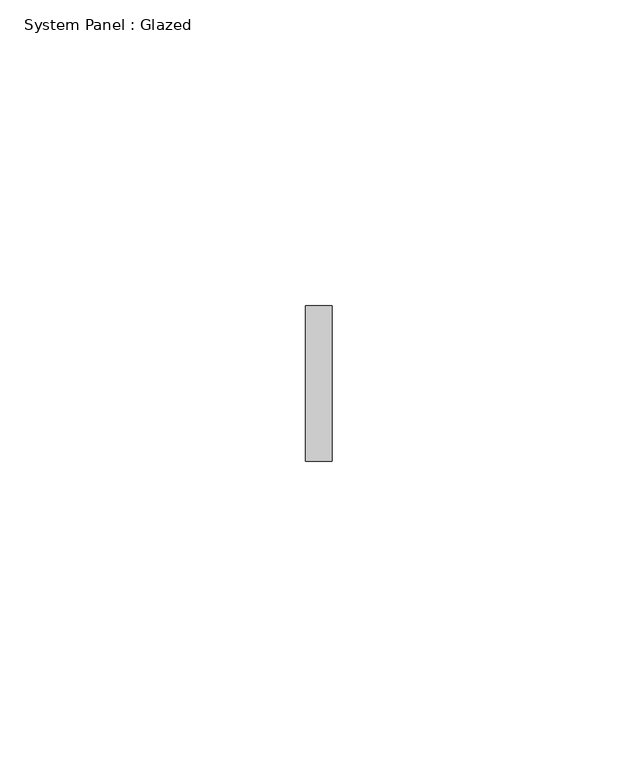
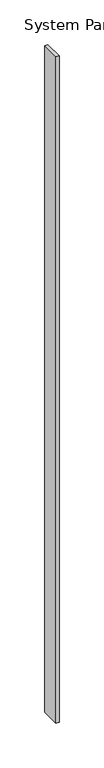
"""IFC4 building model written with IfcOpenShell, lengths in millimetres: plate geometry, System Panel : Glazed."""

from ifc_helpers import new_model, si_unit, origin, origin_with_axes, place, context, project, spatial, polyline, outline, extrude, source, transform, mapped, element, save


def system_panel_glazed_ffe51582(model_context):
    return source(origin(), model_context, "Body", "SweptSolid", [
        extrude(outline(polyline([(2.1789755, 19.05), (-2.1789755, 19.05), (-2.1789755, 44.45), (2.1789755, 44.45), (2.1789755, 19.05)])), origin_with_axes(), (0.0, 0.0, 1.0), 914.4),
    ])


if __name__ == "__main__":
    model = new_model("IFC4")
    model_context = context("Model", 3, world=origin())
    ifc_project = project(units=[si_unit("LENGTHUNIT", "METRE", prefix="MILLI")], contexts=[model_context])
    site = spatial("IfcSite", under=ifc_project)
    building = spatial("IfcBuilding", under=site)
    placement = place(None, origin())
    system_panel_glazed_shape = system_panel_glazed_ffe51582(model_context)
    element("IfcPlate", 1, ObjectType="System Panel : Glazed", at=placement, inside=building, context=model_context, shape_type="MappedRepresentation", body=[
        mapped(system_panel_glazed_shape, transform((0.0, 0.0, 0.0), x_axis=(1.0, 0.0, 0.0), y_axis=(0.0, 1.0, 0.0), z_axis=(0.0, 0.0, 1.0))),
    ])
    save(model, "model.ifc")

# Revit data of these elements
# Type "System Panel : Glazed"
#   Construction Type Id = "GSP4R"
#   Analytic Construction = "1/8 in Pilkington single glazing"
#   Visual Light Transmittance = 0.9
#   Solar Heat Gain Coefficient = 0.86
#   Heat Transfer Coefficient (U) = 6.7069 W/(m²·K)
# Element 1 (IfcPlate, "System Panel : Glazed")
#   Materials on its faces: "Glass"
# Materials
#   "Glass": class "Glass", colour RGB 0 128 192, transparency 0.75, Description = "Soda Lime Glass", Cost = 0
